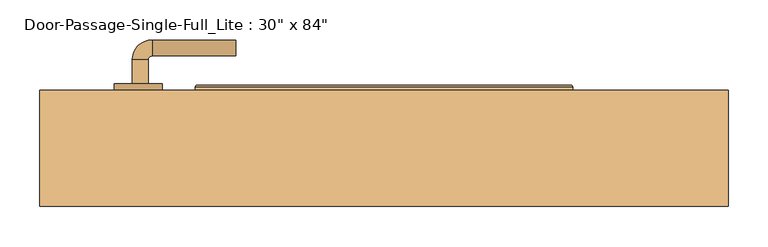
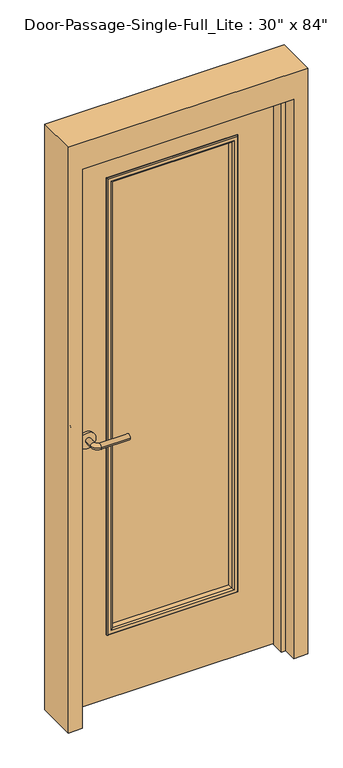
"""IFC4 building model written with IfcOpenShell, lengths in millimetres: door geometry."""

from ifc_helpers import new_model, si_unit, point, frame, frame_2d, origin, place, context, project, spatial, polyline, circle_curve, ellipse_curve, trimmed, segment, composite_curve, outline, extrude, faceted_brep, source, transform, mapped, element, save
from ifc_brep_helpers import plane_surface, cylinder_surface, revolved_surface, advanced_brep


def door_29f5c000(model_context):
    return source(origin(), model_context, "Body", "SolidModel", [
        advanced_brep(
        [(-315.990625, 4.7, 1016.0), (-295.990625, 4.7, 1016.0), (-295.990625, -25.3, 1016.0), (-315.990625, -25.3, 1016.0), (-290.990625, -30.3, 1016.0), (-290.990625, -50.3, 1016.0), (-185.990625, -50.3, 1016.0), (-185.990625, -30.3, 1016.0)],
        [
            (0, 1, circle_curve(frame((-305.990625, 4.7, 1016.0), z_axis=(0.0, 1.0, 0.0), x_axis=(1.0, 0.0, 0.0)), 10.0)),
            (1, 0, circle_curve(frame((-305.990625, 4.7, 1016.0), z_axis=(0.0, 1.0, 0.0), x_axis=(1.0, 0.0, 0.0)), 10.0)),
            (1, 2),
            (2, 3, circle_curve(frame((-305.990625, -25.3, 1016.0), z_axis=(0.0, 1.0, 0.0), x_axis=(1.0, 0.0, 0.0)), 10.0)),
            (3, 0),
            (3, 2, circle_curve(frame((-305.990625, -25.3, 1016.0), z_axis=(0.0, 1.0, 0.0), x_axis=(1.0, 0.0, 0.0)), 10.0)),
            (4, 5, circle_curve(frame((-290.990625, -40.3, 1016.0), z_axis=(-1.0, 0.0, 0.0), x_axis=(0.0, 1.0, 0.0)), 10.0)),
            (5, 3, circle_curve(frame((-290.990625, -25.3, 1016.0), z_axis=(0.0, 0.0, -1.0), x_axis=(-1.0, 0.0, 0.0)), 25.0)),
            (2, 4, circle_curve(frame((-290.990625, -25.3, 1016.0), z_axis=(0.0, 0.0, 1.0), x_axis=(-1.0, 0.0, 0.0)), 5.0)),
            (5, 4, circle_curve(frame((-290.990625, -40.3, 1016.0), z_axis=(-1.0, 0.0, 0.0), x_axis=(0.0, 1.0, 0.0)), 10.0)),
            (6, 7, circle_curve(frame((-185.990625, -40.3, 1016.0), z_axis=(1.0, 0.0, 0.0), x_axis=(0.0, 1.0, 0.0)), 10.0)),
            (7, 6, circle_curve(frame((-185.990625, -40.3, 1016.0), z_axis=(1.0, 0.0, 0.0), x_axis=(0.0, 1.0, 0.0)), 10.0)),
            (4, 7),
            (6, 5),
        ],
        [
            plane_surface(frame((-305.990625, 4.7, 1016.0), z_axis=(0.0, 1.0, 0.0), x_axis=(0.0, 0.0, 1.0))),
            cylinder_surface(frame((-305.990625, 4.7, 1016.0), z_axis=(0.0, 1.0, 0.0), x_axis=(1.0, 0.0, 0.0)), 10.0),
            revolved_surface(trimmed(ellipse_curve(frame((-305.990625, -25.3, 1016.0), z_axis=(0.0, -1.0, 0.0), x_axis=(1.0, 0.0, 0.0)), 10.0, 10.0), [point((-315.990625, -25.3, 1016.0))], [point((-295.990625, -25.3, 1016.0))], True, "CARTESIAN"), (-290.990625, -25.3, 1016.0), (0.0, 0.0, -1.0)),
            revolved_surface(trimmed(ellipse_curve(frame((-305.990625, -25.3, 1016.0), z_axis=(0.0, -1.0, 0.0), x_axis=(1.0, 0.0, 0.0)), 10.0, 10.0), [point((-295.990625, -25.3, 1016.0))], [point((-315.990625, -25.3, 1016.0))], True, "CARTESIAN"), (-290.990625, -25.3, 1016.0), (0.0, 0.0, -1.0)),
            plane_surface(frame((-185.990625, -40.3, 1016.0), z_axis=(1.0, 0.0, 0.0), x_axis=(0.0, 0.0, 1.0))),
            cylinder_surface(frame((-290.990625, -40.3, 1016.0), z_axis=(-1.0, 0.0, 0.0), x_axis=(0.0, 1.0, 0.0)), 10.0),
        ],
        [
            (0, [[1, 2]]),
            (1, [[3, 4, 5, -2]]),
            (1, [[-5, 6, -3, -1]]),
            (2, [[7, 8, -4, 9]]),
            (3, [[10, -9, -6, -8]]),
            (4, [[11, 12]]),
            (5, [[13, -11, 14, -7]]),
            (5, [[-14, -12, -13, -10]]),
        ],
    ),
        extrude(outline(composite_curve([segment(trimmed(circle_curve(frame_2d((1016.0, -308.490625)), 30.0), [point((1016.0, -338.490625))], [point((1016.0, -278.490625))], False, "CARTESIAN"), True, "CONTINUOUS"), segment(trimmed(circle_curve(frame_2d((1016.0, -308.490625)), 30.0), [point((1016.0, -278.490625))], [point((1016.0, -338.490625))], False, "CARTESIAN"), True, "CONTINUOUS")], self_intersect=False)), frame((0.0, 4.7, 0.0), z_axis=(0.0, 1.0, 0.0), x_axis=(0.0, 0.0, 1.0)), (0.0, 0.0, 1.0), 8.0),
        advanced_brep(
        [(-315.990625, 65.15, 1016.0), (-295.990625, 65.15, 1016.0), (-315.990625, 95.15, 1016.0), (-295.990625, 95.15, 1016.0), (-290.990625, 100.15, 1016.0), (-290.990625, 120.15, 1016.0), (-185.990625, 120.15, 1016.0), (-185.990625, 100.15, 1016.0)],
        [
            (0, 1, circle_curve(frame((-305.990625, 65.15, 1016.0), z_axis=(0.0, -1.0, 0.0), x_axis=(1.0, 0.0, 0.0)), 10.0)),
            (1, 0, circle_curve(frame((-305.990625, 65.15, 1016.0), z_axis=(0.0, -1.0, 0.0), x_axis=(1.0, 0.0, 0.0)), 10.0)),
            (0, 2),
            (2, 3, circle_curve(frame((-305.990625, 95.15, 1016.0), z_axis=(0.0, -1.0, 0.0), x_axis=(1.0, 0.0, 0.0)), 10.0)),
            (3, 1),
            (3, 2, circle_curve(frame((-305.990625, 95.15, 1016.0), z_axis=(0.0, -1.0, 0.0), x_axis=(1.0, 0.0, 0.0)), 10.0)),
            (4, 3, circle_curve(frame((-290.990625, 95.15, 1016.0), z_axis=(0.0, 0.0, 1.0), x_axis=(-1.0, 0.0, 0.0)), 5.0)),
            (2, 5, circle_curve(frame((-290.990625, 95.15, 1016.0), z_axis=(0.0, 0.0, -1.0), x_axis=(-1.0, 0.0, 0.0)), 25.0)),
            (5, 4, circle_curve(frame((-290.990625, 110.15, 1016.0), z_axis=(-1.0, 0.0, 0.0), x_axis=(0.0, -1.0, 0.0)), 10.0)),
            (4, 5, circle_curve(frame((-290.990625, 110.15, 1016.0), z_axis=(-1.0, 0.0, 0.0), x_axis=(0.0, -1.0, 0.0)), 10.0)),
            (6, 7, circle_curve(frame((-185.990625, 110.15, 1016.0), z_axis=(1.0, 0.0, 0.0), x_axis=(0.0, -1.0, 0.0)), 10.0)),
            (7, 6, circle_curve(frame((-185.990625, 110.15, 1016.0), z_axis=(1.0, 0.0, 0.0), x_axis=(0.0, -1.0, 0.0)), 10.0)),
            (5, 6),
            (7, 4),
        ],
        [
            plane_surface(frame((-305.990625, 65.15, 1016.0), z_axis=(0.0, -1.0, 0.0), x_axis=(0.0, 0.0, 1.0))),
            cylinder_surface(frame((-305.990625, 65.15, 1016.0), z_axis=(0.0, -1.0, 0.0), x_axis=(1.0, 0.0, 0.0)), 10.0),
            revolved_surface(trimmed(ellipse_curve(frame((-305.990625, 95.15, 1016.0), z_axis=(0.0, -1.0, 0.0), x_axis=(1.0, 0.0, 0.0)), 10.0, 10.0), [point((-315.990625, 95.15, 1016.0))], [point((-295.990625, 95.15, 1016.0))], True, "CARTESIAN"), (-290.990625, 95.15, 1016.0), (0.0, 0.0, -1.0)),
            revolved_surface(trimmed(ellipse_curve(frame((-305.990625, 95.15, 1016.0), z_axis=(0.0, -1.0, 0.0), x_axis=(1.0, 0.0, 0.0)), 10.0, 10.0), [point((-295.990625, 95.15, 1016.0))], [point((-315.990625, 95.15, 1016.0))], True, "CARTESIAN"), (-290.990625, 95.15, 1016.0), (0.0, 0.0, -1.0)),
            plane_surface(frame((-185.990625, 110.15, 1016.0), z_axis=(1.0, 0.0, 0.0), x_axis=(0.0, 0.0, 1.0))),
            cylinder_surface(frame((-290.990625, 110.15, 1016.0), z_axis=(-1.0, 0.0, 0.0), x_axis=(0.0, -1.0, 0.0)), 10.0),
        ],
        [
            (0, [[1, 2]]),
            (1, [[-1, 3, 4, 5]]),
            (1, [[-2, -5, 6, -3]]),
            (2, [[7, -4, 8, 9]]),
            (3, [[-8, -6, -7, 10]]),
            (4, [[11, 12]]),
            (5, [[-9, 13, -12, 14]]),
            (5, [[-10, -14, -11, -13]]),
        ],
    ),
        extrude(outline(composite_curve([segment(trimmed(circle_curve(frame_2d((1016.0, -308.490625)), 30.0), [point((1016.0, -338.490625))], [point((1016.0, -278.490625))], False, "CARTESIAN"), True, "CONTINUOUS"), segment(trimmed(circle_curve(frame_2d((1016.0, -308.490625)), 30.0), [point((1016.0, -278.490625))], [point((1016.0, -338.490625))], False, "CARTESIAN"), True, "CONTINUOUS")], self_intersect=False)), frame((0.0, 57.15, 0.0), z_axis=(0.0, 1.0, 0.0), x_axis=(0.0, 0.0, 1.0)), (0.0, 0.0, 1.0), 8.0),
        extrude(outline(polyline([(228.6, 31.75), (-228.6, 31.75), (-228.6, 38.1), (228.6, 38.1), (228.6, 31.75)])), frame((0.0, 0.0, 254.0), z_axis=(0.0, 0.0, 1.0), x_axis=(1.0, 0.0, 0.0)), (0.0, 0.0, 1.0), 1727.2),
        faceted_brep([(381.0, 7.9375, 0.0), (381.0, 57.15, 0.0), (431.8, 57.15, 0.0), (431.8, -88.9, 0.0), (381.0, -88.9, 0.0), (381.0, -39.6875, 0.0), (365.125, -39.6875, 0.0), (365.125, 7.9375, 0.0), (381.0, 7.9375, 2133.6), (381.0, 57.15, 2133.6), (-381.0, 57.15, 2133.6), (-381.0, 57.15, 0.0), (-431.8, 57.15, 0.0), (-431.8, 57.15, 2235.2), (431.8, 57.15, 2235.2), (431.8, -88.9, 2235.2), (-431.8, -88.9, 2235.2), (-431.8, -88.9, 0.0), (-381.0, -88.9, 0.0), (-381.0, -88.9, 2133.6), (381.0, -88.9, 2133.6), (381.0, -39.6875, 2133.6), (-381.0, -39.6875, 2133.6), (-381.0, -39.6875, 0.0), (-365.125, -39.6875, 0.0), (-365.125, -39.6875, 2117.725), (365.125, -39.6875, 2117.725), (365.125, 7.9375, 2117.725), (-365.125, 7.9375, 2117.725), (-365.125, 7.9375, 0.0), (-381.0, 7.9375, 0.0), (-381.0, 7.9375, 2133.6)], [[[0, 1, 2, 3, 4, 5, 6, 7]], [[1, 0, 8, 9]], [[2, 1, 9, 10, 11, 12, 13, 14]], [[3, 2, 14, 15]], [[4, 3, 15, 16, 17, 18, 19, 20]], [[5, 4, 20, 21]], [[6, 5, 21, 22, 23, 24, 25, 26]], [[7, 6, 26, 27]], [[0, 7, 27, 28, 29, 30, 31, 8]], [[9, 8, 31, 10]], [[20, 19, 22, 21]], [[26, 25, 28, 27]], [[12, 11, 30, 29, 24, 23, 18, 17]], [[11, 10, 31, 30]], [[13, 12, 17, 16]], [[19, 18, 23, 22]], [[25, 24, 29, 28]], [[15, 14, 13, 16]]]),
        extrude(outline(polyline([(2133.6, -381.0), (0.0, -381.0), (0.0, 381.0), (2133.6, 381.0), (2133.6, -381.0)]), holes=[polyline([(1981.2, -228.6), (1981.2, 228.6), (254.0, 228.6), (254.0, -228.6), (1981.2, -228.6)])]), frame((0.0, 12.7, 0.0), z_axis=(0.0, 1.0, 0.0), x_axis=(0.0, 0.0, 1.0)), (0.0, 0.0, 1.0), 44.45),
        advanced_brep(
        [(-228.6, 38.1, 1981.2), (-228.6, 57.15, 1981.2), (-228.6, 57.15, 254.0), (-228.6, 38.1, 254.0), (-216.6, 58.15, 1969.2), (-216.6, 38.1, 1969.2), (-216.6, 38.1, 266.0), (-216.6, 58.15, 266.0), (-221.6, 63.15, 1974.2), (-221.6, 63.15, 261.0), (-236.6, 61.15, 1989.2), (-234.6, 63.15, 1987.2), (-234.6, 63.15, 248.0), (-236.6, 61.15, 246.0), (-236.6, 57.15, 1989.2), (-236.6, 57.15, 246.0), (228.6, 57.15, 254.0), (228.6, 38.1, 254.0), (216.6, 38.1, 266.0), (216.6, 58.15, 266.0), (221.6, 63.15, 261.0), (234.6, 63.15, 248.0), (236.6, 61.15, 246.0), (236.6, 57.15, 246.0), (228.6, 57.15, 1981.2), (228.6, 38.1, 1981.2), (216.6, 38.1, 1969.2), (216.6, 58.15, 1969.2), (221.6, 63.15, 1974.2), (234.6, 63.15, 1987.2), (236.6, 61.15, 1989.2), (236.6, 57.15, 1989.2)],
        [
            (0, 1),
            (1, 2),
            (2, 3),
            (3, 0),
            (4, 5),
            (5, 6),
            (6, 7),
            (7, 4),
            (8, 4, ellipse_curve(frame((-221.6, 58.15, 1974.2), z_axis=(-0.7071067811865475, 0.0, -0.7071067811865475), x_axis=(-0.7071067811865474, 0.0, 0.7071067811865476)), 7.0710678, 5.0)),
            (7, 9, ellipse_curve(frame((-221.6, 58.15, 261.0), z_axis=(-0.7071067811865475, 0.0, 0.7071067811865475), x_axis=(0.7071067811865474, 0.0, 0.7071067811865476)), 7.0710678, 5.0)),
            (9, 8),
            (10, 11, ellipse_curve(frame((-234.6, 61.15, 1987.2), z_axis=(-0.7071067811865475, 0.0, -0.7071067811865475), x_axis=(-0.7071067811865474, 0.0, 0.7071067811865476)), 2.8284271, 2.0)),
            (11, 12),
            (12, 13, ellipse_curve(frame((-234.6, 61.15, 248.0), z_axis=(-0.7071067811865475, 0.0, 0.7071067811865475), x_axis=(0.7071067811865474, 0.0, 0.7071067811865476)), 2.8284271, 2.0)),
            (13, 10),
            (14, 10),
            (13, 15),
            (15, 14),
            (2, 16),
            (16, 17),
            (17, 3),
            (6, 18),
            (18, 19),
            (19, 7),
            (19, 20, ellipse_curve(frame((221.6, 58.15, 261.0), z_axis=(-0.7071067811865475, 0.0, -0.7071067811865475), x_axis=(-0.7071067811865476, 0.0, 0.7071067811865474)), 7.0710678, 5.0)),
            (20, 9),
            (12, 21),
            (21, 22, ellipse_curve(frame((234.6, 61.15, 248.0), z_axis=(-0.7071067811865475, 0.0, -0.7071067811865475), x_axis=(-0.7071067811865476, 0.0, 0.7071067811865474)), 2.8284271, 2.0)),
            (22, 13),
            (22, 23),
            (23, 15),
            (16, 24),
            (24, 25),
            (25, 17),
            (18, 26),
            (26, 27),
            (27, 19),
            (27, 28, ellipse_curve(frame((221.6, 58.15, 1974.2), z_axis=(0.7071067811865475, 0.0, -0.7071067811865475), x_axis=(-0.7071067811865474, 0.0, -0.7071067811865476)), 7.0710678, 5.0)),
            (28, 20),
            (21, 29),
            (29, 30, ellipse_curve(frame((234.6, 61.15, 1987.2), z_axis=(0.7071067811865475, 0.0, -0.7071067811865475), x_axis=(-0.7071067811865474, 0.0, -0.7071067811865476)), 2.8284271, 2.0)),
            (30, 22),
            (30, 31),
            (31, 23),
            (31, 14),
            (1, 24),
            (0, 25),
            (5, 26),
            (4, 27),
            (8, 28),
            (11, 29),
            (10, 30),
        ],
        [
            plane_surface(frame((-228.6, 57.15, 1981.2), z_axis=(-1.0, 0.0, 0.0), x_axis=(0.0, 0.0, -1.0))),
            plane_surface(frame((-216.6, 38.1, 1969.2), z_axis=(1.0, 0.0, 0.0), x_axis=(0.0, 0.0, -1.0))),
            cylinder_surface(frame((-221.6, 58.15, 1981.2), z_axis=(0.0, 0.0, 1.0), x_axis=(-1.0, 0.0, 0.0)), 5.0),
            cylinder_surface(frame((-234.6, 61.15, 1981.2), z_axis=(0.0, 0.0, 1.0), x_axis=(-1.0, 0.0, 0.0)), 2.0),
            plane_surface(frame((-236.6, 61.15, 1989.2), z_axis=(-1.0, 0.0, 0.0), x_axis=(0.0, 0.0, -1.0))),
            plane_surface(frame((-228.6, 57.15, 254.0), z_axis=(0.0, 0.0, -1.0), x_axis=(1.0, 0.0, 0.0))),
            plane_surface(frame((-216.6, 38.1, 266.0), z_axis=(0.0, 0.0, 1.0), x_axis=(1.0, 0.0, 0.0))),
            cylinder_surface(frame((-228.6, 58.15, 261.0), z_axis=(-1.0, 0.0, 0.0), x_axis=(0.0, 0.0, -1.0)), 5.0),
            cylinder_surface(frame((-228.6, 61.15, 248.0), z_axis=(-1.0, 0.0, 0.0), x_axis=(0.0, 0.0, -1.0)), 2.0),
            plane_surface(frame((-236.6, 61.15, 246.0), z_axis=(0.0, 0.0, -1.0), x_axis=(1.0, 0.0, 0.0))),
            plane_surface(frame((228.6, 57.15, 254.0), z_axis=(1.0, 0.0, 0.0), x_axis=(0.0, 0.0, 1.0))),
            plane_surface(frame((216.6, 38.1, 266.0), z_axis=(-1.0, 0.0, 0.0), x_axis=(0.0, 0.0, 1.0))),
            cylinder_surface(frame((221.6, 58.15, 254.0), z_axis=(0.0, 0.0, -1.0), x_axis=(1.0, 0.0, 0.0)), 5.0),
            cylinder_surface(frame((234.6, 61.15, 254.0), z_axis=(0.0, 0.0, -1.0), x_axis=(1.0, 0.0, 0.0)), 2.0),
            plane_surface(frame((236.6, 61.15, 246.0), z_axis=(1.0, 0.0, 0.0), x_axis=(0.0, 0.0, 1.0))),
            plane_surface(frame((236.6, 57.15, 1989.2), z_axis=(0.0, -1.0, 0.0), x_axis=(-1.0, 0.0, 0.0))),
            plane_surface(frame((228.6, 57.15, 1981.2), z_axis=(0.0, 0.0, 1.0), x_axis=(-1.0, 0.0, 0.0))),
            plane_surface(frame((228.6, 38.1, 1981.2), z_axis=(0.0, -1.0, 0.0), x_axis=(-1.0, 0.0, 0.0))),
            plane_surface(frame((216.6, 38.1, 1969.2), z_axis=(0.0, 0.0, -1.0), x_axis=(-1.0, 0.0, 0.0))),
            cylinder_surface(frame((228.6, 58.15, 1974.2), z_axis=(1.0, 0.0, 0.0), x_axis=(0.0, 0.0, 1.0)), 5.0),
            plane_surface(frame((221.6, 63.15, 1974.2), z_axis=(0.0, 1.0, 0.0), x_axis=(-1.0, 0.0, 0.0))),
            cylinder_surface(frame((228.6, 61.15, 1987.2), z_axis=(1.0, 0.0, 0.0), x_axis=(0.0, 0.0, 1.0)), 2.0),
            plane_surface(frame((236.6, 61.15, 1989.2), z_axis=(0.0, 0.0, 1.0), x_axis=(-1.0, 0.0, 0.0))),
        ],
        [
            (0, [[1, 2, 3, 4]]),
            (1, [[5, 6, 7, 8]]),
            (2, [[9, -8, 10, 11]]),
            (3, [[12, 13, 14, 15]]),
            (4, [[16, -15, 17, 18]]),
            (5, [[-3, 19, 20, 21]]),
            (6, [[-7, 22, 23, 24]]),
            (7, [[-10, -24, 25, 26]]),
            (8, [[-14, 27, 28, 29]]),
            (9, [[-17, -29, 30, 31]]),
            (10, [[-20, 32, 33, 34]]),
            (11, [[-23, 35, 36, 37]]),
            (12, [[-25, -37, 38, 39]]),
            (13, [[-28, 40, 41, 42]]),
            (14, [[-30, -42, 43, 44]]),
            (15, [[-31, -44, 45, -18], [46, -32, -19, -2]]),
            (16, [[-33, -46, -1, 47]]),
            (17, [[-21, -34, -47, -4], [48, -35, -22, -6]]),
            (18, [[-36, -48, -5, 49]]),
            (19, [[-38, -49, -9, 50]]),
            (20, [[51, -40, -27, -13], [-26, -39, -50, -11]]),
            (21, [[-41, -51, -12, 52]]),
            (22, [[-43, -52, -16, -45]]),
        ],
    ),
        advanced_brep(
        [(-228.6, 31.75, 254.0), (-228.6, 12.7, 254.0), (-228.6, 12.7, 1981.2), (-228.6, 31.75, 1981.2), (-216.6, 11.7, 266.0), (-216.6, 31.75, 266.0), (-216.6, 31.75, 1969.2), (-216.6, 11.7, 1969.2), (-221.6, 6.7, 261.0), (-221.6, 6.7, 1974.2), (-236.6, 8.7, 246.0), (-234.6, 6.7, 248.0), (-234.6, 6.7, 1987.2), (-236.6, 8.7, 1989.2), (-236.6, 12.7, 246.0), (-236.6, 12.7, 1989.2), (228.6, 12.7, 1981.2), (228.6, 31.75, 1981.2), (216.6, 31.75, 1969.2), (216.6, 11.7, 1969.2), (221.6, 6.7, 1974.2), (234.6, 6.7, 1987.2), (236.6, 8.7, 1989.2), (236.6, 12.7, 1989.2), (228.6, 12.7, 254.0), (228.6, 31.75, 254.0), (216.6, 31.75, 266.0), (216.6, 11.7, 266.0), (221.6, 6.7, 261.0), (234.6, 6.7, 248.0), (236.6, 8.7, 246.0), (236.6, 12.7, 246.0)],
        [
            (0, 1),
            (1, 2),
            (2, 3),
            (3, 0),
            (4, 5),
            (5, 6),
            (6, 7),
            (7, 4),
            (8, 4, ellipse_curve(frame((-221.6, 11.7, 261.0), z_axis=(-0.7071067811865475, 0.0, 0.7071067811865475), x_axis=(-0.7071067811865474, 0.0, -0.7071067811865476)), 7.0710678, 5.0)),
            (7, 9, ellipse_curve(frame((-221.6, 11.7, 1974.2), z_axis=(-0.7071067811865475, 0.0, -0.7071067811865475), x_axis=(0.7071067811865474, 0.0, -0.7071067811865476)), 7.0710678, 5.0)),
            (9, 8),
            (10, 11, ellipse_curve(frame((-234.6, 8.7, 248.0), z_axis=(-0.7071067811865475, 0.0, 0.7071067811865475), x_axis=(-0.7071067811865474, 0.0, -0.7071067811865476)), 2.8284271, 2.0)),
            (11, 12),
            (12, 13, ellipse_curve(frame((-234.6, 8.7, 1987.2), z_axis=(-0.7071067811865475, 0.0, -0.7071067811865475), x_axis=(0.7071067811865474, 0.0, -0.7071067811865476)), 2.8284271, 2.0)),
            (13, 10),
            (14, 10),
            (13, 15),
            (15, 14),
            (2, 16),
            (16, 17),
            (17, 3),
            (6, 18),
            (18, 19),
            (19, 7),
            (19, 20, ellipse_curve(frame((221.6, 11.7, 1974.2), z_axis=(-0.7071067811865475, 0.0, 0.7071067811865475), x_axis=(-0.7071067811865476, 0.0, -0.7071067811865474)), 7.0710678, 5.0)),
            (20, 9),
            (12, 21),
            (21, 22, ellipse_curve(frame((234.6, 8.7, 1987.2), z_axis=(-0.7071067811865475, 0.0, 0.7071067811865475), x_axis=(-0.7071067811865476, 0.0, -0.7071067811865474)), 2.8284271, 2.0)),
            (22, 13),
            (22, 23),
            (23, 15),
            (16, 24),
            (24, 25),
            (25, 17),
            (18, 26),
            (26, 27),
            (27, 19),
            (27, 28, ellipse_curve(frame((221.6, 11.7, 261.0), z_axis=(0.7071067811865475, 0.0, 0.7071067811865475), x_axis=(-0.7071067811865474, 0.0, 0.7071067811865476)), 7.0710678, 5.0)),
            (28, 20),
            (21, 29),
            (29, 30, ellipse_curve(frame((234.6, 8.7, 248.0), z_axis=(0.7071067811865475, 0.0, 0.7071067811865475), x_axis=(-0.7071067811865474, 0.0, 0.7071067811865476)), 2.8284271, 2.0)),
            (30, 22),
            (30, 31),
            (31, 23),
            (31, 14),
            (1, 24),
            (0, 25),
            (5, 26),
            (4, 27),
            (8, 28),
            (11, 29),
            (10, 30),
        ],
        [
            plane_surface(frame((-228.6, 12.7, 254.0), z_axis=(-1.0, 0.0, 0.0), x_axis=(0.0, 0.0, 1.0))),
            plane_surface(frame((-216.6, 31.75, 266.0), z_axis=(1.0, 0.0, 0.0), x_axis=(0.0, 0.0, 1.0))),
            cylinder_surface(frame((-221.6, 11.7, 254.0), z_axis=(0.0, 0.0, -1.0), x_axis=(-1.0, 0.0, 0.0)), 5.0),
            cylinder_surface(frame((-234.6, 8.7, 254.0), z_axis=(0.0, 0.0, -1.0), x_axis=(-1.0, 0.0, 0.0)), 2.0),
            plane_surface(frame((-236.6, 8.7, 246.0), z_axis=(-1.0, 0.0, 0.0), x_axis=(0.0, 0.0, 1.0))),
            plane_surface(frame((-228.6, 12.7, 1981.2), z_axis=(0.0, 0.0, 1.0), x_axis=(1.0, 0.0, 0.0))),
            plane_surface(frame((-216.6, 31.75, 1969.2), z_axis=(0.0, 0.0, -1.0), x_axis=(1.0, 0.0, 0.0))),
            cylinder_surface(frame((-228.6, 11.7, 1974.2), z_axis=(-1.0, 0.0, 0.0), x_axis=(0.0, 0.0, 1.0)), 5.0),
            cylinder_surface(frame((-228.6, 8.7, 1987.2), z_axis=(-1.0, 0.0, 0.0), x_axis=(0.0, 0.0, 1.0)), 2.0),
            plane_surface(frame((-236.6, 8.7, 1989.2), z_axis=(0.0, 0.0, 1.0), x_axis=(1.0, 0.0, 0.0))),
            plane_surface(frame((228.6, 12.7, 1981.2), z_axis=(1.0, 0.0, 0.0), x_axis=(0.0, 0.0, -1.0))),
            plane_surface(frame((216.6, 31.75, 1969.2), z_axis=(-1.0, 0.0, 0.0), x_axis=(0.0, 0.0, -1.0))),
            cylinder_surface(frame((221.6, 11.7, 1981.2), z_axis=(0.0, 0.0, 1.0), x_axis=(1.0, 0.0, 0.0)), 5.0),
            cylinder_surface(frame((234.6, 8.7, 1981.2), z_axis=(0.0, 0.0, 1.0), x_axis=(1.0, 0.0, 0.0)), 2.0),
            plane_surface(frame((236.6, 8.7, 1989.2), z_axis=(1.0, 0.0, 0.0), x_axis=(0.0, 0.0, -1.0))),
            plane_surface(frame((236.6, 12.7, 246.0), z_axis=(0.0, 1.0, 0.0), x_axis=(-1.0, 0.0, 0.0))),
            plane_surface(frame((228.6, 12.7, 254.0), z_axis=(0.0, 0.0, -1.0), x_axis=(-1.0, 0.0, 0.0))),
            plane_surface(frame((228.6, 31.75, 254.0), z_axis=(0.0, 1.0, 0.0), x_axis=(-1.0, 0.0, 0.0))),
            plane_surface(frame((216.6, 31.75, 266.0), z_axis=(0.0, 0.0, 1.0), x_axis=(-1.0, 0.0, 0.0))),
            cylinder_surface(frame((228.6, 11.7, 261.0), z_axis=(1.0, 0.0, 0.0), x_axis=(0.0, 0.0, -1.0)), 5.0),
            plane_surface(frame((221.6, 6.7, 261.0), z_axis=(0.0, -1.0, 0.0), x_axis=(-1.0, 0.0, 0.0))),
            cylinder_surface(frame((228.6, 8.7, 248.0), z_axis=(1.0, 0.0, 0.0), x_axis=(0.0, 0.0, -1.0)), 2.0),
            plane_surface(frame((236.6, 8.7, 246.0), z_axis=(0.0, 0.0, -1.0), x_axis=(-1.0, 0.0, 0.0))),
        ],
        [
            (0, [[1, 2, 3, 4]]),
            (1, [[5, 6, 7, 8]]),
            (2, [[9, -8, 10, 11]]),
            (3, [[12, 13, 14, 15]]),
            (4, [[16, -15, 17, 18]]),
            (5, [[-3, 19, 20, 21]]),
            (6, [[-7, 22, 23, 24]]),
            (7, [[-10, -24, 25, 26]]),
            (8, [[-14, 27, 28, 29]]),
            (9, [[-17, -29, 30, 31]]),
            (10, [[-20, 32, 33, 34]]),
            (11, [[-23, 35, 36, 37]]),
            (12, [[-25, -37, 38, 39]]),
            (13, [[-28, 40, 41, 42]]),
            (14, [[-30, -42, 43, 44]]),
            (15, [[-31, -44, 45, -18], [46, -32, -19, -2]]),
            (16, [[-33, -46, -1, 47]]),
            (17, [[-21, -34, -47, -4], [48, -35, -22, -6]]),
            (18, [[-36, -48, -5, 49]]),
            (19, [[-38, -49, -9, 50]]),
            (20, [[51, -40, -27, -13], [-26, -39, -50, -11]]),
            (21, [[-41, -51, -12, 52]]),
            (22, [[-43, -52, -16, -45]]),
        ],
    ),
    ])


if __name__ == "__main__":
    model = new_model("IFC4")
    model_context = context("Model", 3, world=origin())
    ifc_project = project(units=[si_unit("LENGTHUNIT", "METRE", prefix="MILLI")], contexts=[model_context])
    site = spatial("IfcSite", under=ifc_project)
    building = spatial("IfcBuilding", under=site)
    placement = place(None, origin())
    door_shape = door_29f5c000(model_context)
    element("IfcDoor", 1, ObjectType="Door-Passage-Single-Full_Lite : 30\" x 84\"", at=placement, inside=building, context=model_context, shape_type="MappedRepresentation", body=[
        mapped(door_shape, transform((0.0, 0.0, 0.0), x_axis=(1.0, 0.0, 0.0), y_axis=(0.0, 1.0, 0.0), z_axis=(0.0, 0.0, 1.0))),
    ])
    save(model, "model.ifc")

# Revit data of these elements
# Type "Door-Passage-Single-Full_Lite : 30\" x 84\""
#   Type Mark = "9"
#   Assembly Code = "B2030100"
#   Analytic Construction = "Wooden"
#   Thickness = 0' - 1 3/4"
#   Thermal Resistance (R) = 2.5876 (h·ft²·°F)/BTU
#   Swing Angle [instance default] = 90.00°
#   Strike Height = 3' - 4"
#   Rough Width [instance default] = 2' - 10"
#   Rough Height [instance default] = 7' - 4"
#   MF Opening Height [instance default] = 0' - 4"
#   MF Opening Width [instance default] = 0' - 4"
#   Inset Calculate [instance default] = 0' - 4"
#   Masonry Inset [instance default] = 0' - 1"
#   Height = 7' - 0"
#   Width = 2' - 6"
#   Heat Transfer Coefficient (U) = 0.3865 BTU/(h·ft²·°F)
#   Masonry Frame Depth = 0' - 5 3/4"
#   Masonry Frame [instance default] = yes
#   Function = 1
#   Dry Wall Frame [instance default] = no
#   Panel Material = Wood - Birch
#   Glazing = Glass
#   Glass Stop Material = Metal - Paint Finish - Grey
#   Frame Material = Metal - Paint Finish - Grey
#   Door Handle Material = Aluminum
#   Visual Light Transmittance = 0
#   Solar Heat Gain Coefficient = 0
#   Wall Closure = (empty or 0)
# Element 1 (IfcDoor, "Door-Passage-Single-Full_Lite : 30\" x 84\"")
#   Materials on its faces: "Metal - Paint Finish - Grey", "Aluminum", "Wood - Birch", "Glass"
# Materials
#   "Wood - Birch": class "Wood", colour RGB 166 116 52, transparency 0, Cost = 0
#   "Glass": class "Glass", colour RGB 0 128 192, transparency 0.75, Description = "Soda Lime Glass", Cost = 0
#   "Metal - Paint Finish - Grey": class "Paint", colour RGB 104 104 104, transparency 0, Cost = 0
#   "Aluminum": class "Metal", colour RGB 247 247 247, transparency 0, Description = "Aluminum 6061", Cost = 0
